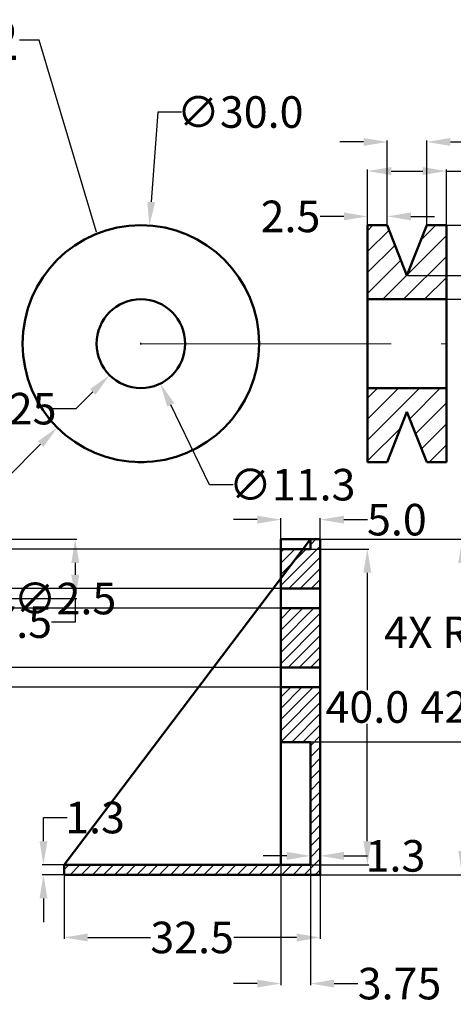
# Model space of a CAD drawing. Units: inches. Extents: x 0 to 231, y -13 to 111.
# Tile 2 of 3: x 83 to 138, y -13 to 111. Entities that reach past the tile are written whole.
import ezdxf
from ezdxf import colors
from ezdxf.entities.mleader import LeaderData, LeaderLine
from ezdxf.math import Vec2, Vec3

# ---------------------------------------------------------------- set-up
doc = ezdxf.new("R2010")
doc.units = ezdxf.units.IN
doc.header["$MEASUREMENT"] = 0
doc.linetypes.add('CENTER', pattern=[50.8, 31.75, -6.35, 6.35, -6.35])
for name, color, linetype, lineweight in [('M-CNTR', 1, 'CENTER', 18), ('M-DIMS', 2, 'Continuous', 25), ('M-HATC', 8, 'Continuous', 18), ('M-OUTL', 7, 'Continuous', 50), ('M-TEXT', 3, 'Continuous', 25)]:
    doc.layers.add(name, color=color, linetype=linetype, lineweight=lineweight)
doc.styles.get("Standard").update_dxf_attribs({"font": 'arial.ttf'})
doc.dimstyles.get("Standard").update_dxf_attribs({"dimtxt": 4, "dimasz": 3, "dimexe": 0.18, "dimexo": 0.0625, "dimgap": 0.09, "dimtad": 0, "dimtih": 1, "dimtoh": 1, "dimdec": 1, "dimzin": 0, "dimdsep": 46, "dimtxsty": 'Standard', "dimcen": 0.09, "dimadec": 0, "dimazin": 0, "dimtfac": 1, "dimtdec": 1, "dimtofl": 0, "dimtmove": 0, "dimatfit": 3, "dimfxl": 1, "dimtolj": 1, "dimtzin": 0, "dimarcsym": 0})

# ---------------------------------------------------------------- blocks, each defined once
blk = doc.blocks.new('*D6')
at = {"layer": 'Defpoints', "color": 0, "transparency": 16777216}
for p in [(126.95, 86.33), (126.95, 85.21), (129.45, 85.21)]:
    blk.add_point(p, dxfattribs=at)
at = {"layer": 'M-DIMS', "color": 0, "lineweight": -2, "transparency": 16777216}
for p, q in [((123.95, 86.33), (120.95, 86.33)), ((126.95, 85.27), (126.95, 86.51)), ((129.45, 85.27), (129.45, 86.51)), ((132.45, 86.33), (135.45, 86.33))]:
    blk.add_line(p, q, dxfattribs=at)
at = {"layer": 'M-DIMS', "color": 0, "transparency": 16777216}
for points in [[(123.95, 86.83), (123.95, 85.83), (126.95, 86.33)], [(132.45, 86.83), (132.45, 85.83), (129.45, 86.33)]]:
    blk.add_solid(points, dxfattribs=at)
at = {"layer": 'M-DIMS', "color": 0, "transparency": 16777216, "insert": (117.17, 86.33), "char_height": 4, "attachment_point": 5}
blk.add_mtext('\\A1;2.5', dxfattribs=at)
blk = doc.blocks.new('*D7')
at = {"layer": 'Defpoints', "color": 0, "transparency": 16777216}
for p in [(136.95, 92.07), (126.95, 85.21), (136.95, 85.21)]:
    blk.add_point(p, dxfattribs=at)
at = {"layer": 'M-DIMS', "color": 0, "lineweight": -2, "transparency": 16777216}
for p, q in [((126.95, 85.27), (126.95, 92.25)), ((129.95, 92.07), (133.95, 92.07)), ((136.95, 85.27), (136.95, 92.25)), ((136.95, 92.07), (139.95, 92.07))]:
    blk.add_line(p, q, dxfattribs=at)
at = {"layer": 'M-DIMS', "color": 0, "transparency": 16777216}
for points in [[(129.95, 92.57), (129.95, 91.57), (126.95, 92.07)], [(133.95, 92.57), (133.95, 91.57), (136.95, 92.07)]]:
    blk.add_solid(points, dxfattribs=at)
at = {"layer": 'M-DIMS', "color": 0, "transparency": 16777216, "insert": (145.04, 92.07), "char_height": 4, "attachment_point": 5}
blk.add_mtext('\\A1;10.0', dxfattribs=at)
blk = doc.blocks.new('*D8')
at = {"layer": 'Defpoints', "color": 0, "transparency": 16777216}
for p in [(99.28, 85.17), (97.1, 55.25)]:
    blk.add_point(p, dxfattribs=at)
at = {"layer": 'M-DIMS', "color": 0, "lineweight": -2, "transparency": 16777216}
for p, q in [((100.33, 99.55), (99.5, 88.16)), ((103.33, 99.55), (100.33, 99.55)), ((98.1, 70.21), (98.28, 70.21)), ((98.19, 70.12), (98.19, 70.3))]:
    blk.add_line(p, q, dxfattribs=at)
at = {"layer": 'M-DIMS', "color": 0, "transparency": 16777216}
blk.add_solid([(99, 88.2), (100, 88.13), (99.28, 85.17)], dxfattribs=at)
at = {"layer": 'M-DIMS', "color": 0, "transparency": 16777216, "insert": (110.79, 99.55), "char_height": 4, "attachment_point": 5}
blk.add_mtext('\\A1;∅30.0', dxfattribs=at)
blk = doc.blocks.new('*D9')
at = {"layer": 'Defpoints', "color": 0, "transparency": 16777216}
for p in [(95.72, 75.26), (100.66, 65.16)]:
    blk.add_point(p, dxfattribs=at)
at = {"layer": 'M-DIMS', "color": 0, "lineweight": -2, "transparency": 16777216}
for p, q in [((98.1, 70.21), (98.28, 70.21)), ((98.19, 70.12), (98.19, 70.3)), ((106.92, 52.35), (101.98, 62.46)), ((109.92, 52.35), (106.92, 52.35))]:
    blk.add_line(p, q, dxfattribs=at)
at = {"layer": 'M-DIMS', "color": 0, "transparency": 16777216}
blk.add_solid([(102.43, 62.68), (101.53, 62.24), (100.66, 65.16)], dxfattribs=at)
at = {"layer": 'M-DIMS', "color": 0, "transparency": 16777216, "insert": (117.38, 52.35), "char_height": 4, "attachment_point": 5}
blk.add_mtext('\\A1;∅11.3', dxfattribs=at)
blk = doc.blocks.new('*D13')
at = {"layer": 'Defpoints', "color": 0, "transparency": 16777216}
for p in [(67.47, 45.44), (67.47, 37.94), (89.87, 37.94)]:
    blk.add_point(p, dxfattribs=at)
at = {"layer": 'M-DIMS', "color": 0, "lineweight": -2, "transparency": 16777216}
for p, q in [((67.53, 45.44), (90.05, 45.44)), ((89.87, 42.44), (89.87, 40.94)), ((67.53, 37.94), (90.05, 37.94)), ((89.87, 37.94), (89.87, 34.94)), ((89.87, 34.94), (86.87, 34.94))]:
    blk.add_line(p, q, dxfattribs=at)
at = {"layer": 'M-DIMS', "color": 0, "transparency": 16777216}
for points in [[(89.37, 42.44), (90.37, 42.44), (89.87, 45.44)], [(89.37, 40.94), (90.37, 40.94), (89.87, 37.94)]]:
    blk.add_solid(points, dxfattribs=at)
at = {"layer": 'M-DIMS', "color": 0, "transparency": 16777216, "insert": (83.14, 34.94), "char_height": 4, "attachment_point": 5}
blk.add_mtext('\\A1;7.5', dxfattribs=at)
blk = doc.blocks.new('*D14')
at = {"layer": 'Defpoints', "color": 0, "transparency": 16777216}
for p in [(85.84, 4.19), (88.45, 4.19), (88.45, 2.94)]:
    blk.add_point(p, dxfattribs=at)
at = {"layer": 'M-DIMS', "color": 0, "lineweight": -2, "transparency": 16777216}
for p, q in [((85.84, 7.19), (85.84, 10.19)), ((85.84, 10.19), (88.84, 10.19)), ((88.38, 4.19), (85.66, 4.19)), ((88.38, 2.94), (85.66, 2.94)), ((85.84, -0.06), (85.84, -3.06))]:
    blk.add_line(p, q, dxfattribs=at)
at = {"layer": 'M-DIMS', "color": 0, "transparency": 16777216}
for points in [[(85.34, 7.19), (86.34, 7.19), (85.84, 4.19)], [(85.34, -0.06), (86.34, -0.06), (85.84, 2.94)]]:
    blk.add_solid(points, dxfattribs=at)
at = {"layer": 'M-DIMS', "color": 0, "transparency": 16777216, "insert": (92.38, 10.19), "char_height": 4, "attachment_point": 5}
blk.add_mtext('\\A1;1.3', dxfattribs=at)
blk = doc.blocks.new('*D15')
at = {"layer": 'Defpoints', "color": 0, "transparency": 16777216}
for p in [(88.45, 2.94), (120.95, 2.94), (120.95, -5)]:
    blk.add_point(p, dxfattribs=at)
at = {"layer": 'M-DIMS', "color": 0, "lineweight": -2, "transparency": 16777216}
for p, q in [((88.45, 2.88), (88.45, -5.18)), ((120.95, 2.88), (120.95, -5.18)), ((91.45, -5), (99.4, -5)), ((117.95, -5), (110, -5))]:
    blk.add_line(p, q, dxfattribs=at)
at = {"layer": 'M-DIMS', "color": 0, "transparency": 16777216}
for points in [[(91.45, -4.5), (91.45, -5.5), (88.45, -5)], [(117.95, -4.5), (117.95, -5.5), (120.95, -5)]]:
    blk.add_solid(points, dxfattribs=at)
at = {"layer": 'M-DIMS', "color": 0, "transparency": 16777216, "insert": (104.7, -5), "char_height": 4, "attachment_point": 5}
blk.add_mtext('\\A1;32.5', dxfattribs=at)
blk = doc.blocks.new('*D16')
at = {"layer": 'Defpoints', "color": 0, "transparency": 16777216}
for p in [(120.95, 5.34), (119.7, 4.92), (120.95, 4.92)]:
    blk.add_point(p, dxfattribs=at)
at = {"layer": 'M-DIMS', "color": 0, "lineweight": -2, "transparency": 16777216}
for p, q in [((116.7, 5.34), (113.7, 5.34)), ((119.7, 4.98), (119.7, 5.52)), ((120.95, 4.98), (120.95, 5.52)), ((123.95, 5.34), (126.95, 5.34))]:
    blk.add_line(p, q, dxfattribs=at)
at = {"layer": 'M-DIMS', "color": 0, "transparency": 16777216}
for points in [[(116.7, 5.84), (116.7, 4.84), (119.7, 5.34)], [(123.95, 5.84), (123.95, 4.84), (120.95, 5.34)]]:
    blk.add_solid(points, dxfattribs=at)
at = {"layer": 'M-DIMS', "color": 0, "transparency": 16777216, "insert": (130.49, 5.34), "char_height": 4, "attachment_point": 5}
blk.add_mtext('\\A1;1.3', dxfattribs=at)
blk = doc.blocks.new('*D17')
at = {"layer": 'Defpoints', "color": 0, "transparency": 16777216}
for p in [(120.95, 45.44), (120.95, 2.94), (138.96, 2.94)]:
    blk.add_point(p, dxfattribs=at)
at = {"layer": 'M-DIMS', "color": 0, "lineweight": -2, "transparency": 16777216}
for p, q in [((121.01, 45.44), (139.14, 45.44)), ((138.96, 42.44), (138.96, 26.33)), ((138.96, 5.94), (138.96, 22.06)), ((121.01, 2.94), (139.14, 2.94))]:
    blk.add_line(p, q, dxfattribs=at)
at = {"layer": 'M-DIMS', "color": 0, "transparency": 16777216}
for points in [[(138.46, 42.44), (139.46, 42.44), (138.96, 45.44)], [(138.46, 5.94), (139.46, 5.94), (138.96, 2.94)]]:
    blk.add_solid(points, dxfattribs=at)
at = {"layer": 'M-DIMS', "color": 0, "transparency": 16777216, "insert": (138.96, 24.19), "char_height": 4, "attachment_point": 5}
blk.add_mtext('\\A1;42.5', dxfattribs=at)
blk = doc.blocks.new('*D18')
at = {"layer": 'Defpoints', "color": 0, "transparency": 16777216}
for p in [(119.7, 44.19), (119.7, 4.19), (126.92, 4.19)]:
    blk.add_point(p, dxfattribs=at)
at = {"layer": 'M-DIMS', "color": 0, "lineweight": -2, "transparency": 16777216}
for p, q in [((119.76, 44.19), (127.1, 44.19)), ((126.92, 41.19), (126.92, 26.33)), ((126.92, 7.19), (126.92, 22.06)), ((119.76, 4.19), (127.1, 4.19))]:
    blk.add_line(p, q, dxfattribs=at)
at = {"layer": 'M-DIMS', "color": 0, "transparency": 16777216}
for points in [[(126.42, 41.19), (127.42, 41.19), (126.92, 44.19)], [(126.42, 7.19), (127.42, 7.19), (126.92, 4.19)]]:
    blk.add_solid(points, dxfattribs=at)
at = {"layer": 'M-DIMS', "color": 0, "transparency": 16777216, "insert": (126.92, 24.19), "char_height": 4, "attachment_point": 5}
blk.add_mtext('\\A1;40.0', dxfattribs=at)
blk = doc.blocks.new('*D19')
at = {"layer": 'Defpoints', "color": 0, "transparency": 16777216}
for p in [(120.95, 47.92), (115.95, 45.44), (120.95, 45.44)]:
    blk.add_point(p, dxfattribs=at)
at = {"layer": 'M-DIMS', "color": 0, "lineweight": -2, "transparency": 16777216}
for p, q in [((112.95, 47.92), (109.95, 47.92)), ((115.95, 45.51), (115.95, 48.1)), ((120.95, 45.51), (120.95, 48.1)), ((123.95, 47.92), (126.95, 47.92))]:
    blk.add_line(p, q, dxfattribs=at)
at = {"layer": 'M-DIMS', "color": 0, "transparency": 16777216}
for points in [[(112.95, 48.42), (112.95, 47.42), (115.95, 47.92)], [(123.95, 48.42), (123.95, 47.42), (120.95, 47.92)]]:
    blk.add_solid(points, dxfattribs=at)
at = {"layer": 'M-DIMS', "color": 0, "transparency": 16777216, "insert": (130.67, 47.92), "char_height": 4, "attachment_point": 5}
blk.add_mtext('\\A1;5.0', dxfattribs=at)
blk = doc.blocks.new('*D34')
at = {"layer": 'Defpoints', "color": 0, "transparency": 16777216}
for p in [(134.45, 95.76), (129.45, 85.21), (134.45, 85.21)]:
    blk.add_point(p, dxfattribs=at)
at = {"layer": 'M-DIMS', "color": 0, "lineweight": -2, "transparency": 16777216}
for p, q in [((126.45, 95.76), (123.45, 95.76)), ((129.45, 85.27), (129.45, 95.94)), ((134.45, 85.27), (134.45, 95.94)), ((137.45, 95.76), (140.45, 95.76))]:
    blk.add_line(p, q, dxfattribs=at)
at = {"layer": 'M-DIMS', "color": 0, "transparency": 16777216}
for points in [[(126.45, 96.26), (126.45, 95.26), (129.45, 95.76)], [(137.45, 96.26), (137.45, 95.26), (134.45, 95.76)]]:
    blk.add_solid(points, dxfattribs=at)
at = {"layer": 'M-DIMS', "color": 0, "transparency": 16777216, "insert": (144.17, 95.76), "char_height": 4, "attachment_point": 5}
blk.add_mtext('\\A1;5.0', dxfattribs=at)
blk = doc.blocks.new('*D35')
at = {"layer": 'Defpoints', "color": 0, "transparency": 16777216}
for p in [(136.95, 85.21), (214.08, 85.21), (131.95, 78.84)]:
    blk.add_point(p, dxfattribs=at)
at = {"layer": 'M-DIMS', "color": 0, "lineweight": -2, "transparency": 16777216}
for p, q in [((214.08, 85.21), (214.08, 88.21)), ((214.08, 88.21), (217.08, 88.21)), ((137.01, 85.21), (214.26, 85.21)), ((214.08, 81.84), (214.08, 82.21)), ((132.01, 78.84), (214.26, 78.84))]:
    blk.add_line(p, q, dxfattribs=at)
at = {"layer": 'M-DIMS', "color": 0, "transparency": 16777216}
for points in [[(213.58, 82.21), (214.58, 82.21), (214.08, 85.21)], [(213.58, 81.84), (214.58, 81.84), (214.08, 78.84)]]:
    blk.add_solid(points, dxfattribs=at)
at = {"layer": 'M-DIMS', "color": 0, "transparency": 16777216, "insert": (223.94, 88.21), "char_height": 4, "attachment_point": 5}
blk.add_mtext('\\A1;6.375', dxfattribs=at)
blk = doc.blocks.new('*D36')
at = {"layer": 'Defpoints', "color": 0, "transparency": 16777216}
for p in [(136.95, 85.21), (136.95, 75.84), (214.08, 75.84)]:
    blk.add_point(p, dxfattribs=at)
at = {"layer": 'M-DIMS', "color": 0, "lineweight": -2, "transparency": 16777216}
for p, q in [((137.01, 85.21), (214.26, 85.21)), ((214.08, 82.21), (214.08, 78.84)), ((137.01, 75.84), (214.26, 75.84)), ((214.08, 75.84), (214.08, 72.84)), ((214.08, 72.84), (211.08, 72.84))]:
    blk.add_line(p, q, dxfattribs=at)
at = {"layer": 'M-DIMS', "color": 0, "transparency": 16777216}
for points in [[(213.58, 82.21), (214.58, 82.21), (214.08, 85.21)], [(213.58, 78.84), (214.58, 78.84), (214.08, 75.84)]]:
    blk.add_solid(points, dxfattribs=at)
at = {"layer": 'M-DIMS', "color": 0, "transparency": 16777216, "insert": (204.22, 72.84), "char_height": 4, "attachment_point": 5}
blk.add_mtext('\\A1;9.375', dxfattribs=at)
blk = doc.blocks.new('*D41')
at = {"layer": 'Defpoints', "color": 0, "transparency": 16777216}
for p in [(115.946436, 44.192783), (13.844426, 39.192783), (115.946436, 39.192783)]:
    blk.add_point(p, dxfattribs=at)
at = {"layer": 'M-DIMS', "color": 0, "lineweight": -2, "transparency": 16777216}
for p, q in [((13.844426, 47.192783), (13.844426, 50.192783)), ((115.883936, 44.192783), (13.664426, 44.192783)), ((115.883936, 39.192783), (13.664426, 39.192783)), ((13.844426, 36.192783), (13.844426, 33.192783))]:
    blk.add_line(p, q, dxfattribs=at)
at = {"layer": 'M-DIMS', "color": 0, "transparency": 16777216}
for points in [[(13.344426, 47.192783), (14.344426, 47.192783), (13.844426, 44.192783)], [(13.344426, 36.192783), (14.344426, 36.192783), (13.844426, 39.192783)]]:
    blk.add_solid(points, dxfattribs=at)
at = {"layer": 'M-DIMS', "color": 0, "transparency": 16777216, "insert": (13.844426, 41.692783), "char_height": 4, "attachment_point": 5}
blk.add_mtext('\\A1;5.0', dxfattribs=at)
blk = doc.blocks.new('*D42')
at = {"layer": 'Defpoints', "color": 0, "transparency": 16777216}
for p in [(115.95, 39.19), (13.84, 36.69), (115.95, 36.69)]:
    blk.add_point(p, dxfattribs=at)
at = {"layer": 'M-DIMS', "color": 0, "lineweight": -2, "transparency": 16777216}
for p, q in [((13.84, 42.19), (13.84, 45.19)), ((115.88, 39.19), (13.66, 39.19)), ((115.88, 36.69), (13.66, 36.69)), ((13.84, 33.69), (13.84, 30.69)), ((13.84, 30.69), (10.84, 30.69))]:
    blk.add_line(p, q, dxfattribs=at)
at = {"layer": 'M-DIMS', "color": 0, "transparency": 16777216}
for points in [[(13.34, 42.19), (14.34, 42.19), (13.84, 39.19)], [(13.34, 33.69), (14.34, 33.69), (13.84, 36.69)]]:
    blk.add_solid(points, dxfattribs=at)
at = {"layer": 'M-DIMS', "color": 0, "transparency": 16777216, "insert": (7.06, 30.69), "char_height": 4, "attachment_point": 5}
blk.add_mtext('\\A1;2.5', dxfattribs=at)
blk = doc.blocks.new('*D43')
at = {"layer": 'Defpoints', "color": 0, "transparency": 16777216}
for p in [(115.95, 36.69), (13.84, 29.19), (115.95, 29.19)]:
    blk.add_point(p, dxfattribs=at)
at = {"layer": 'M-DIMS', "color": 0, "lineweight": -2, "transparency": 16777216}
for p, q in [((115.88, 36.69), (13.66, 36.69)), ((13.84, 33.69), (13.84, 32.19)), ((115.88, 29.19), (13.66, 29.19)), ((13.84, 29.19), (13.84, 26.19)), ((13.84, 26.19), (10.84, 26.19))]:
    blk.add_line(p, q, dxfattribs=at)
at = {"layer": 'M-DIMS', "color": 0, "transparency": 16777216}
for points in [[(13.34, 33.69), (14.34, 33.69), (13.84, 36.69)], [(13.34, 32.19), (14.34, 32.19), (13.84, 29.19)]]:
    blk.add_solid(points, dxfattribs=at)
at = {"layer": 'M-DIMS', "color": 0, "transparency": 16777216, "insert": (7.11, 26.19), "char_height": 4, "attachment_point": 5}
blk.add_mtext('\\A1;7.5', dxfattribs=at)
blk = doc.blocks.new('*D44')
at = {"layer": 'Defpoints', "color": 0, "transparency": 16777216}
for p in [(115.95, 29.19), (13.84, 26.69), (115.95, 26.69)]:
    blk.add_point(p, dxfattribs=at)
at = {"layer": 'M-DIMS', "color": 0, "lineweight": -2, "transparency": 16777216}
for p, q in [((13.84, 32.19), (13.84, 35.19)), ((115.88, 29.19), (13.66, 29.19)), ((115.88, 26.69), (13.66, 26.69)), ((13.84, 23.69), (13.84, 20.69)), ((13.84, 20.69), (10.84, 20.69))]:
    blk.add_line(p, q, dxfattribs=at)
at = {"layer": 'M-DIMS', "color": 0, "transparency": 16777216}
for points in [[(13.34, 32.19), (14.34, 32.19), (13.84, 29.19)], [(13.34, 23.69), (14.34, 23.69), (13.84, 26.69)]]:
    blk.add_solid(points, dxfattribs=at)
at = {"layer": 'M-DIMS', "color": 0, "transparency": 16777216, "insert": (7.06, 20.69), "char_height": 4, "attachment_point": 5}
blk.add_mtext('\\A1;2.5', dxfattribs=at)
blk = doc.blocks.new('*D45')
at = {"layer": 'Defpoints', "color": 0, "transparency": 16777216}
for p in [(119.7, 19.76), (120.95, 2.94), (214.08, 2.94)]:
    blk.add_point(p, dxfattribs=at)
at = {"layer": 'M-DIMS', "color": 0, "lineweight": -2, "transparency": 16777216}
for p, q in [((119.76, 19.76), (214.26, 19.76)), ((214.08, 16.76), (214.08, 13.48)), ((214.08, 5.94), (214.08, 9.22)), ((121.01, 2.94), (214.26, 2.94))]:
    blk.add_line(p, q, dxfattribs=at)
at = {"layer": 'M-DIMS', "color": 0, "transparency": 16777216}
for points in [[(213.58, 16.76), (214.58, 16.76), (214.08, 19.76)], [(213.58, 5.94), (214.58, 5.94), (214.08, 2.94)]]:
    blk.add_solid(points, dxfattribs=at)
at = {"layer": 'M-DIMS', "color": 0, "transparency": 16777216, "insert": (214.08, 11.35), "char_height": 4, "attachment_point": 5}
blk.add_mtext('\\A1;16.816', dxfattribs=at)
blk = doc.blocks.new('*D46')
at = {"layer": 'Defpoints', "color": 0, "transparency": 16777216}
for p in [(115.95, 19.76), (119.7, 19.76), (119.7, -10.84)]:
    blk.add_point(p, dxfattribs=at)
at = {"layer": 'M-DIMS', "color": 0, "lineweight": -2, "transparency": 16777216}
for p, q in [((115.95, 19.7), (115.95, -11.02)), ((119.7, 19.7), (119.7, -11.02)), ((112.95, -10.84), (109.95, -10.84)), ((122.7, -10.84), (125.7, -10.84))]:
    blk.add_line(p, q, dxfattribs=at)
at = {"layer": 'M-DIMS', "color": 0, "transparency": 16777216}
for points in [[(112.95, -10.34), (112.95, -11.34), (115.95, -10.84)], [(122.7, -10.34), (122.7, -11.34), (119.7, -10.84)]]:
    blk.add_solid(points, dxfattribs=at)
at = {"layer": 'M-DIMS', "color": 0, "transparency": 16777216, "insert": (131, -10.84), "char_height": 4, "attachment_point": 5}
blk.add_mtext('\\A1;3.75', dxfattribs=at)
blk = doc.blocks.new('*D51')
at = {"layer": 'Defpoints', "color": 0, "transparency": 16777216}
for p in [(108.79, 80.83), (87.6, 59.6)]:
    blk.add_point(p, dxfattribs=at)
at = {"layer": 'M-DIMS', "color": 0, "lineweight": -2, "transparency": 16777216}
for p, q in [((98.1, 70.21), (98.28, 70.21)), ((98.19, 70.12), (98.19, 70.3)), ((81.24, 53.23), (85.48, 57.47)), ((78.24, 53.23), (81.24, 53.23))]:
    blk.add_line(p, q, dxfattribs=at)
at = {"layer": 'M-DIMS', "color": 0, "transparency": 16777216}
blk.add_solid([(85.12, 57.83), (85.83, 57.12), (87.6, 59.6)], dxfattribs=at)
at = {"layer": 'M-DIMS', "color": 0, "transparency": 16777216, "insert": (70.78, 53.23), "char_height": 4, "attachment_point": 5}
blk.add_mtext('\\A1;∅30.0', dxfattribs=at)
blk = doc.blocks.new('*D52')
at = {"layer": 'Defpoints', "color": 0, "transparency": 16777216}
for p in [(102.17, 74.19), (94.22, 66.23)]:
    blk.add_point(p, dxfattribs=at)
at = {"layer": 'M-DIMS', "color": 0, "lineweight": -2, "transparency": 16777216}
for p, q in [((98.1, 70.21), (98.28, 70.21)), ((98.19, 70.12), (98.19, 70.3)), ((89.98, 61.98), (92.1, 64.11)), ((86.98, 61.98), (89.98, 61.98))]:
    blk.add_line(p, q, dxfattribs=at)
at = {"layer": 'M-DIMS', "color": 0, "transparency": 16777216}
blk.add_solid([(91.75, 64.46), (92.45, 63.75), (94.22, 66.23)], dxfattribs=at)
at = {"layer": 'M-DIMS', "color": 0, "transparency": 16777216, "insert": (77.95, 61.98), "char_height": 4, "attachment_point": 5}
blk.add_mtext('\\A1;∅11.25', dxfattribs=at)
blk = doc.blocks.new('*D54')
at = {"layer": 'Defpoints', "color": 0, "transparency": 16777216}
for p in [(66.22, 37.95), (68.72, 37.94)]:
    blk.add_point(p, dxfattribs=at)
at = {"layer": 'M-DIMS', "color": 0, "lineweight": -2, "transparency": 16777216}
for p, q in [((67.38, 37.94), (67.56, 37.94)), ((67.47, 37.85), (67.47, 38.03)), ((74.72, 37.93), (71.72, 37.93))]:
    blk.add_line(p, q, dxfattribs=at)
at = {"layer": 'M-DIMS', "color": 0, "transparency": 16777216}
blk.add_solid([(71.72, 38.43), (71.72, 37.43), (68.72, 37.94)], dxfattribs=at)
at = {"layer": 'M-DIMS', "color": 0, "transparency": 16777216, "insert": (84.87, 37.93), "char_height": 4, "attachment_point": 5}
blk.add_mtext('\\A1;2X ∅2.5', dxfattribs=at)
blk = doc.blocks.new('*D58')
at = {"layer": 'Defpoints', "color": 0, "transparency": 16777216}
for p in [(157.75, 27.66), (157.91, 25.07)]:
    blk.add_point(p, dxfattribs=at)
at = {"layer": 'M-DIMS', "color": 0, "lineweight": -2, "transparency": 16777216}
for p, q in [((154.39, 33.65), (157.39, 33.65)), ((157.39, 33.65), (157.57, 30.65)), ((157.82, 25.07), (158, 25.07)), ((157.91, 24.98), (157.91, 25.16))]:
    blk.add_line(p, q, dxfattribs=at)
at = {"layer": 'M-DIMS', "color": 0, "transparency": 16777216}
blk.add_solid([(158.07, 30.68), (157.07, 30.62), (157.75, 27.66)], dxfattribs=at)
at = {"layer": 'M-DIMS', "color": 0, "transparency": 16777216, "insert": (141.28, 33.65), "char_height": 4, "attachment_point": 5}
blk.add_mtext('\\A1;4X R2.592', dxfattribs=at)

msp = doc.modelspace()

# ---------------------------------------------------------------- hatches: boundary and pattern name
at = {"layer": 'M-HATC'}
h = msp.add_hatch(dxfattribs=at)
h.set_pattern_fill('ANSI31', color=256, scale=15)
h.paths.add_polyline_path([(136.9483, 85.2103), (134.4483, 85.2103), (131.9483, 78.8353), (129.4483, 85.2103), (126.9483, 85.2103), (126.9483, 75.8353), (136.9483, 75.8353)])
h.paths.add_polyline_path([(136.9483, 64.5853), (126.9483, 64.5853), (126.9483, 55.2156), (129.4483, 55.2156), (131.9483, 61.5853), (134.4483, 55.2156), (136.9483, 55.2156)])
h = msp.add_hatch(dxfattribs=at)
h.set_pattern_fill('ANSI31', color=256, scale=8)
h.paths.add_polyline_path([(120.9464, 26.6928), (115.9464, 26.6928), (115.9464, 19.7587), (119.6964, 19.7587), (119.6964, 4.1928), (88.4464, 4.1928), (88.4464, 2.9428), (120.9464, 2.9428)])
h.paths.add_polyline_path([(120.9464, 45.4428), (119.6964, 45.4428), (119.6964, 44.1928), (118.7495, 44.1928), (115.9464, 40.4928), (115.9464, 39.1928), (120.9464, 39.1928)])
h.paths.add_polyline_path([(118.7495, 44.1928), (115.9464, 44.1928), (115.9464, 40.4928)], flags=17)
h.paths.add_polyline_path([(120.9464, 36.6928), (115.9464, 36.6928), (115.9464, 29.1928), (120.9464, 29.1928)])

# ---------------------------------------------------------------- linework, layer by layer
at = {"layer": 'M-CNTR'}
msp.add_line((98.1935, 70.2103), (136.9483, 70.2103), dxfattribs=at)
at = {"layer": 'M-OUTL'}
for p, q in [((126.9483, 85.2103), (129.4483, 85.2103)), ((126.9483, 85.2103), (126.9483, 55.2156)), ((129.4483, 85.2103), (131.9483, 78.8353)), ((131.9483, 78.8353), (134.4483, 85.2103)), ((134.4483, 85.2103), (136.9483, 85.2103)), ((136.9483, 85.2103), (136.9483, 55.2156)), ((126.9483, 75.8353), (136.9483, 75.8353)), ((126.9483, 64.5853), (136.9483, 64.5853)), ((129.4483, 55.2156), (131.9483, 61.5853)), ((131.9483, 61.5853), (134.4483, 55.2156)), ((97.7931, 55.2156), (98.5939, 55.2156)), ((126.9483, 55.2156), (129.4483, 55.2156)), ((134.4483, 55.2156), (136.9483, 55.2156)), ((119.6964, 45.4428), (88.4464, 4.1928)), ((120.9464, 45.4428), (115.9464, 45.4428)), ((115.9464, 45.4428), (115.9464, 4.1928)), ((119.6964, 44.1928), (119.6964, 45.4428)), ((120.9464, 2.9428), (120.9464, 45.4428)), ((115.9464, 44.1928), (119.6964, 44.1928)), ((115.9464, 39.1928), (120.9464, 39.1928)), ((115.9464, 36.6928), (120.9464, 36.6928)), ((115.9464, 29.1928), (120.9464, 29.1928)), ((115.9464, 26.6928), (120.9464, 26.6928)), ((115.9464, 19.7587), (119.6964, 19.7587)), ((119.6964, 4.1928), (119.6964, 19.7587)), ((88.4464, 4.1928), (119.6964, 4.1928)), ((88.4464, 2.9428), (88.4464, 4.1928)), ((88.4464, 2.9428), (120.9464, 2.9428))]:
    msp.add_line(p, q, dxfattribs=at)
for radius in [15, 5.625]:
    msp.add_circle((98.1935, 70.2103), radius, dxfattribs=at)

# ---------------------------------------------------------------- dimensions: what is measured, and where the dimension line sits
at = {"layer": 'M-DIMS'}
for p1, p2, override, picture, middle in [((97.1029, 55.25), (99.2841, 85.1706), {"dimclrd": 0, "dimclre": 0, "dimclrt": 0}, '*D8', (110.7867, 99.5511)), ((108.7917, 80.8252), (87.5953, 59.5953), {"dimdec": 1, "dimlfac": 1, "dimrnd": 0, "dimzin": 0, "dimdsep": 46, "dimlunit": 2}, '*D51', (70.7821, 53.2263)), ((95.7249, 75.2646), (100.6621, 65.1559), {"dimclrd": 0, "dimclre": 0, "dimclrt": 0}, '*D9', (117.3797, 52.3463)), ((102.1676, 74.1911), (94.2194, 66.2294), {"dimdec": 2, "dimlfac": 1, "dimrnd": 0, "dimzin": 0, "dimdsep": 46, "dimlunit": 2}, '*D52', (77.9504, 61.9832))]:
    dim = msp.add_diameter_dim_2p(p1=p1, p2=p2, dimstyle='Standard', override=override, dxfattribs=at)
    dim.commit()
    dim.dimension.update_dxf_attribs({"geometry": picture, "text_midpoint": middle, "dimtype": 163})
for base, p1, p2, override, picture, middle in [((134.4483, 95.7603), (129.4483, 85.2103), (134.4483, 85.2103), {"dimdec": 1, "dimlfac": 1, "dimrnd": 0, "dimzin": 0, "dimdsep": 46, "dimlunit": 2}, '*D34', (144.1727, 95.7603)), ((136.9483, 92.0651), (126.9483, 85.2103), (136.9483, 85.2103), {"dimclrd": 0, "dimclre": 0, "dimclrt": 0}, '*D7', (145.0383, 92.0651)), ((126.9483, 86.3305), (129.4483, 85.2103), (126.9483, 85.2103), {"dimclrd": 0, "dimclre": 0, "dimclrt": 0}, '*D6', (117.168, 86.3305)), ((120.9464, 47.9192), (115.9464, 45.4428), (120.9464, 45.4428), {"dimclrd": 0, "dimclre": 0, "dimclrt": 0}, '*D19', (130.6708, 47.9192)), ((119.6964, -10.8388), (115.9464, 19.7587), (119.6964, 19.7587), {"dimdec": 2, "dimlfac": 1, "dimrnd": 0, "dimzin": 0, "dimdsep": 46, "dimlunit": 2}, '*D46', (130.9952, -10.8388)), ((120.9464357729, 5.3423703269), (119.6964357729, 4.9165791613), (120.9464357729, 4.9165791613), {"dimclrd": 0, "dimclre": 0, "dimclrt": 0}, '*D16', (130.4893689243, 5.3423703269)), ((120.9464, -5.0008), (88.4464, 2.9428), (120.9464, 2.9428), {"dimclrd": 0, "dimclre": 0, "dimclrt": 0}, '*D15', (104.6964, -5.0008))]:
    dim = msp.add_linear_dim(base=base, p1=p1, p2=p2, dimstyle='Standard', override=override, dxfattribs=at)
    dim.commit()
    dim.dimension.update_dxf_attribs({"geometry": picture, "text_midpoint": middle})
for base, p1, p2, override, picture, middle in [((214.0757, 85.2103), (131.9483, 78.8353), (136.9483, 85.2103), {"dimdec": 3, "dimlfac": 1, "dimrnd": 0, "dimzin": 0, "dimdsep": 46, "dimlunit": 2}, '*D35', (223.9406, 88.2103)), ((214.0757, 75.8353), (136.9483, 85.2103), (136.9483, 75.8353), {"dimdec": 3, "dimlfac": 1, "dimrnd": 0, "dimzin": 0, "dimdsep": 46, "dimlunit": 2}, '*D36', (204.2217, 72.8353)), ((13.8444, 39.1928), (115.9464, 44.1928), (115.9464, 39.1928), {"dimdec": 1, "dimlfac": 1, "dimrnd": 0, "dimzin": 0, "dimdsep": 46, "dimlunit": 2}, '*D41', (13.8444, 41.6928)), ((13.8444, 36.6928), (115.9464, 39.1928), (115.9464, 36.6928), {"dimdec": 1, "dimlfac": 1, "dimrnd": 0, "dimzin": 0, "dimdsep": 46, "dimlunit": 2}, '*D42', (7.0641, 30.6928)), ((89.8714, 37.9428), (67.4708, 45.4428), (67.4708, 37.9428), {"dimclrd": 0, "dimclre": 0, "dimclrt": 0}, '*D13', (83.1415, 34.9428)), ((138.9616, 2.9428), (120.9464, 45.4428), (120.9464, 2.9428), {"dimclrd": 0, "dimclre": 0, "dimclrt": 0}, '*D17', (138.9616, 24.1928)), ((126.9227, 4.1928), (119.6964, 44.1928), (119.6964, 4.1928), {"dimclrd": 0, "dimclre": 0, "dimclrt": 0}, '*D18', (126.9227, 24.1928)), ((13.8444, 29.1928), (115.9464, 36.6928), (115.9464, 29.1928), {"dimdec": 1, "dimlfac": 1, "dimrnd": 0, "dimzin": 0, "dimdsep": 46, "dimlunit": 2}, '*D43', (7.1146, 26.1928)), ((13.8444, 26.6928), (115.9464, 29.1928), (115.9464, 26.6928), {"dimdec": 1, "dimlfac": 1, "dimrnd": 0, "dimzin": 0, "dimdsep": 46, "dimlunit": 2}, '*D44', (7.0641, 20.6928)), ((214.0757, 2.9428), (119.6964, 19.7587), (120.9464, 2.9428), {"dimdec": 3, "dimlfac": 1, "dimrnd": 0, "dimzin": 0, "dimdsep": 46, "dimlunit": 2}, '*D45', (214.0757, 11.3508)), ((85.8350326307, 4.1927826383), (88.4464357729, 2.9427826383), (88.4464357729, 4.1927826383), {"dimclrd": 0, "dimclre": 0, "dimclrt": 0}, '*D14', (92.3779657822, 10.1927826383))]:
    dim = msp.add_linear_dim(base=base, p1=p1, p2=p2, angle=90, dimstyle='Standard', override=override, dxfattribs=at)
    dim.commit()
    dim.dimension.update_dxf_attribs({"geometry": picture, "text_midpoint": middle})
dim = msp.add_diameter_dim_2p(p1=(66.2208, 37.9456), p2=(68.7208, 37.94), text='2X <>', dimstyle='Standard', override={"dimdec": 1, "dimlfac": 1, "dimrnd": 0, "dimzin": 0, "dimdsep": 46, "dimlunit": 2}, dxfattribs=at)
dim.commit()
dim.dimension.update_dxf_attribs({"geometry": '*D54', "text_midpoint": (74.7208, 37.9266)})
dim = msp.add_radius_dim(center=(157.9054, 25.0724), mpoint=(157.75, 27.66), text='4X <>', dimstyle='Standard', override={"dimdec": 3, "dimlfac": 1, "dimrnd": 0, "dimzin": 0, "dimdsep": 46, "dimlunit": 2}, dxfattribs=at)
dim.commit()
dim.dimension.update_dxf_attribs({"geometry": '*D58', "text_midpoint": (141.2799, 33.6492)})

# ---------------------------------------------------------------- leaders
at = {"layer": 'M-TEXT'}
ml = msp.add_multileader_mtext('Standard', dxfattribs=at)
ml.set_content('2', color=256)
ml.set_leader_properties()
ml.build(insert=Vec2(0, 0))
ml.multileader.update_dxf_attribs({"dogleg_length": 0.36, "arrow_head_size": 0.18})
ctx = ml.context
ctx.base_point, ctx.char_height, ctx.arrow_head_size, ctx.landing_gap_size, ctx.plane_origin = Vec3(79.2964, 108.6563), 5, 0.18, 0.09, Vec3(92.632, 84.1412)
ctx.text_align_type = 2
notes = []
notes.append((ctx, [(0, (1, 1, 0), (85.2943, 108.6563), (-1, 0), 2.5062, [(0, [(92.632, 84.1412)], 0, [])])]))
ctx.mtext.insert, ctx.mtext.alignment, ctx.mtext.flow_direction = Vec3(82.6981, 111.1563), 3, 5
for ctx, leaders in notes:
    for number, flags, end, landing, length, lines in leaders:
        leader = LeaderData()
        leader.index, (leader.has_last_leader_line, leader.has_dogleg_vector, leader.attachment_direction) = number, flags
        leader.last_leader_point, leader.dogleg_vector, leader.dogleg_length = Vec3(end), Vec3(landing), length
        for number, points, colour, breaks in lines:
            line = LeaderLine()
            line.index, line.vertices, line.color, line.breaks = number, Vec3.list(points), colors.encode_raw_color(colour), breaks
            leader.lines.append(line)
        ctx.leaders.append(leader)

doc.saveas('drawing.dxf')
